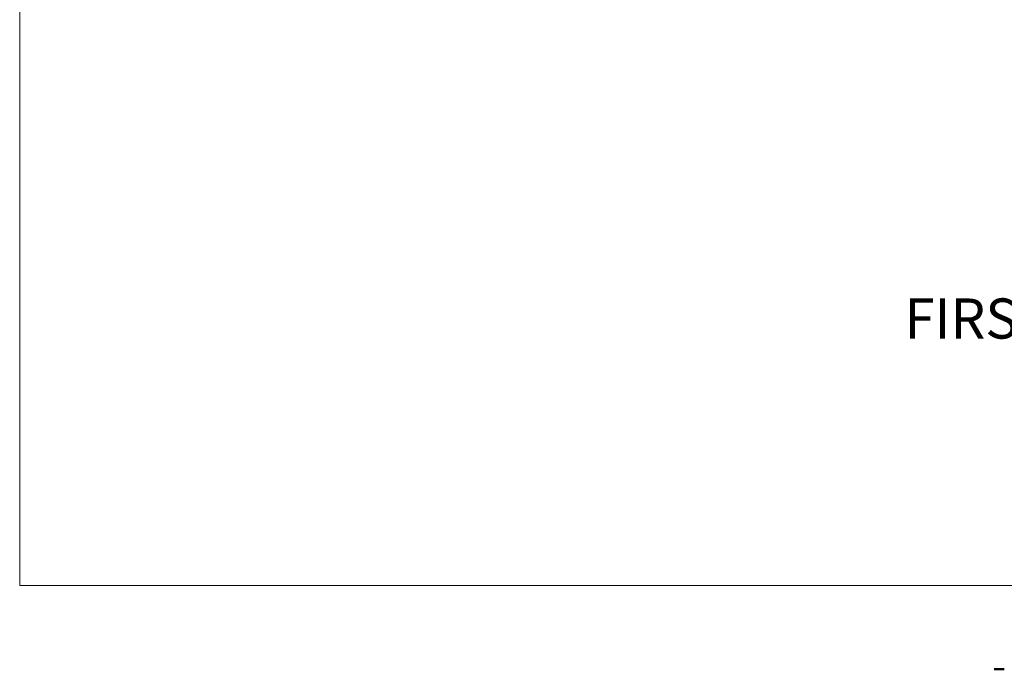
# Model space of a CAD drawing. Units: inches. Extents: x 1901 to 2863, y 888 to 2433.
# Tile 1 of 91: x 1901 to 2343, y 924 to 1216. Entities that reach past the tile are written whole.
import ezdxf

# ---------------------------------------------------------------- set-up
doc = ezdxf.new("R2010")
doc.units = ezdxf.units.IN
for name, color, linetype, lineweight in [('A-ANNO-TEXT', 7, 'Continuous', 35), ('A-FLOR-FIXT', 9, 'Continuous', 18), ('A-WALL', 7, 'Continuous', 50), ('A-WALL-PATT', 8, 'Continuous', 13)]:
    doc.layers.add(name, color=color, linetype=linetype, lineweight=lineweight)
doc.styles.get("Standard").update_dxf_attribs({"font": 'arial.ttf'})

msp = doc.modelspace()

# ---------------------------------------------------------------- hatches: boundary and pattern name
at = {"layer": 'A-WALL-PATT'}
h = msp.add_hatch(dxfattribs=at)
h.set_pattern_fill('ANSI32', color=256)
h.paths.add_polyline_path([(2192.5, 2274.13), (2141.26, 2274.13), (2141.26, 2269.63), (2192.5, 2269.63)])
h.paths.add_polyline_path([(2259.93, 2274.13), (2216.5, 2274.13), (2216.5, 2269.63), (2255.43, 2269.63), (2255.43, 2214.63), (2250.81, 2214.63), (2250.81, 2210.13), (2259.93, 2210.13), (2259.93, 2215.13), (2271.76, 2215.13), (2271.76, 2217.38), (2271.76, 2219.63), (2259.93, 2219.63)])
h.paths.add_polyline_path([(2171.43, 2269.63), (2166.93, 2269.63), (2166.93, 2219.63), (2121.24, 2219.63), (2121.24, 2215.13), (2166.93, 2215.13), (2166.93, 2083.13), (2161.81, 2083.13), (2161.81, 2078.63), (2171.43, 2078.63), (2177, 2078.63), (2177, 2080.88), (2177, 2083.13), (2171.43, 2083.13), (2171.43, 2210.13), (2230.91, 2210.13), (2230.91, 2212.38), (2230.91, 2214.63), (2171.43, 2214.63)])
h.paths.add_polyline_path([(2117.26, 2274.13), (2089.43, 2274.13), (2089.43, 2219.63), (2081.14, 2219.63), (2081.14, 2215.13), (2089.43, 2215.13), (2098, 2215.13), (2098, 2217.38), (2098, 2219.63), (2093.93, 2219.63), (2093.93, 2269.63), (2117.26, 2269.63), (2117.26, 2271.88)])
h.paths.add_polyline_path([(2343.43, 2219.63), (2329.29, 2219.63), (2329.29, 2215.13), (2338.93, 2215.13), (2338.93, 2184.74), (2343.43, 2184.74)])
h.paths.add_polyline_path([(2338.93, 2083.13), (2329.29, 2083.13), (2208.97, 2083.13), (2208.97, 2078.63), (2338.93, 2078.63)])
h.paths.add_polyline_path([(2343.43, 2136.74), (2338.93, 2136.74), (2338.93, 1872.63), (2343.43, 1872.63)])
h.paths.add_polyline_path([(2343.43, 1863.63), (2397.68, 1863.63), (2397.68, 1821.63), (2384.14, 1821.63), (2384.14, 1812.63), (2418.33, 1812.63), (2418.33, 1817.13), (2418.33, 1821.63), (2406.68, 1821.63), (2406.68, 1863.63), (2459.5, 1863.63), (2459.5, 1821.63), (2447.14, 1821.63), (2447.14, 1812.63), (2459.5, 1812.63), (2468.5, 1812.63), (2468.5, 1872.63), (2394.43, 1872.63), (2334.43, 1872.63), (2334.43, 1812.63), (2343.43, 1812.63), (2353.25, 1812.63), (2353.25, 1821.63), (2343.43, 1821.63)])
h.paths.add_polyline_path([(2510.01, 1872.63), (2468.5, 1872.63), (2468.5, 1868.13), (2510.01, 1868.13)])
h.paths.add_polyline_path([(2514.01, 1817.13), (2468.5, 1817.13), (2468.5, 1812.63), (2482.11, 1812.63), (2482.11, 1800.61), (2486.61, 1800.61), (2486.61, 1812.63), (2514.01, 1812.63)])
h.paths.add_polyline_path([(2299.25, 1814.88), (2299.25, 1817.13), (2295.93, 1817.13), (2295.93, 1854.17), (2293.68, 1854.17), (2291.43, 1854.17), (2291.43, 1817.13), (2266.11, 1817.13), (2266.11, 1812.63), (2299.25, 1812.63)])
h.paths.add_polyline_path([(2218.11, 1817.13), (2206.46, 1817.13), (2171.43, 1817.13), (2171.43, 1949.13), (2190.1, 1949.13), (2190.1, 1953.63), (2163.47, 1953.63), (2163.47, 1949.13), (2166.93, 1949.13), (2166.93, 1817.13), (2114.3, 1817.13), (2114.3, 1812.63), (2218.11, 1812.63)])
h.paths.add_polyline_path([(2029.43, 1970.92), (2024.93, 1970.92), (2024.93, 1912.72), (2029.43, 1912.72)])
h.paths.add_polyline_path([(2132.3, 1953.63), (2113.93, 1953.63), (2113.93, 1975.89), (2111.68, 1975.89), (2109.43, 1975.89), (2109.43, 1953.63), (2029.43, 1953.63), (2029.43, 1949.13), (2132.3, 1949.13)])
h.paths.add_polyline_path([(2029.43, 1853.61), (2029.31, 1853.61), (2029.31, 1853.61), (2029.43, 1853.61), (2029.43, 1864.72), (2024.93, 1864.72), (2024.93, 1812.63), (2066.3, 1812.63), (2066.3, 1814.88), (2066.3, 1817.13), (2029.43, 1817.13)])
h.paths.add_polyline_path([(2122.93, 2010.09), (2120.68, 2010.09), (2118.43, 2010.09), (2118.43, 2006.13), (2029.43, 2006.13), (2029.43, 2001.63), (2109.43, 2001.63), (2109.43, 1998.04), (2113.93, 1998.04), (2113.93, 2001.63), (2122.93, 2001.63)])
h.paths.add_polyline_path([(2029.43, 2031.38), (2024.93, 2031.38), (2024.93, 1994.92), (2027.18, 1994.92), (2029.43, 1994.92)])
h.paths.add_polyline_path([(2029.43, 2136.74), (2024.93, 2136.74), (2024.93, 2067.38), (2027.18, 2067.38), (2029.43, 2067.38)])
h.paths.add_polyline_path([(2125.62, 2083.13), (2029.43, 2083.13), (2029.43, 2078.63), (2118.43, 2078.63), (2118.43, 2030.71), (2122.93, 2030.71), (2122.93, 2078.63), (2125.62, 2078.63)])
h.paths.add_polyline_path([(2029.43, 2215.13), (2040.47, 2215.13), (2040.47, 2217.38), (2040.47, 2219.63), (2024.93, 2219.63), (2024.93, 2184.74), (2029.43, 2184.74), (2029.43, 2187.78)])
h.paths.add_polyline_path([(2686.43, 2274.13), (2659.28, 2274.13), (2659.28, 2269.63), (2681.93, 2269.63), (2681.93, 2219.63), (2676.82, 2219.63), (2676.82, 2215.13), (2681.93, 2215.13), (2697.01, 2215.13), (2697.01, 2217.38), (2697.01, 2219.63), (2686.43, 2219.63)])
h.paths.add_polyline_path([(2609.93, 2269.63), (2635.28, 2269.63), (2635.28, 2274.13), (2571.43, 2274.13), (2571.43, 2269.63), (2605.43, 2269.63), (2605.43, 2214.63), (2549.1, 2214.63), (2549.1, 2210.13), (2605.43, 2210.13), (2605.43, 2083.13), (2601.01, 2083.13), (2601.01, 2080.88), (2601.01, 2078.63), (2609.93, 2078.63), (2616.16, 2078.63), (2616.16, 2080.88), (2616.16, 2083.13), (2609.93, 2083.13), (2609.93, 2215.13), (2651.46, 2215.13), (2651.46, 2217.38), (2651.46, 2219.63), (2609.93, 2219.63)])
h.paths.add_polyline_path([(2521.43, 2269.63), (2547.43, 2269.63), (2547.43, 2271.88), (2547.43, 2274.13), (2516.93, 2274.13), (2516.93, 2219.63), (2506.41, 2219.63), (2506.41, 2215.13), (2516.93, 2215.13), (2516.93, 2210.13), (2525.4, 2210.13), (2525.4, 2212.38), (2525.4, 2214.63), (2521.43, 2214.63)])
h.paths.add_polyline_path([(2456.01, 2219.63), (2439.43, 2219.63), (2439.43, 2187.89), (2443.93, 2187.89), (2443.93, 2215.13), (2456.01, 2215.13)])
h.paths.add_polyline_path([(2752.93, 2219.63), (2739.48, 2219.63), (2739.48, 2215.13), (2748.43, 2215.13), (2748.43, 2187.89), (2752.93, 2187.89)])
h.paths.add_polyline_path([(2752.93, 2139.89), (2748.43, 2139.89), (2748.43, 2083.13), (2648.42, 2083.13), (2648.42, 2078.63), (2654.93, 2078.63), (2654.93, 2039.44), (2659.43, 2039.44), (2659.43, 2078.63), (2748.43, 2078.63), (2748.43, 2063.43), (2752.93, 2063.43)])
h.paths.add_polyline_path([(2752.93, 2010.63), (2659.43, 2010.63), (2659.43, 2015.65), (2654.93, 2015.65), (2654.93, 2010.63), (2605.43, 2010.63), (2605.43, 1920.97), (2609.93, 1920.97), (2609.93, 2006.13), (2748.43, 2006.13), (2748.43, 1982.47), (2752.93, 1982.47)])
h.paths.add_polyline_path([(2752.93, 2027.43), (2748.43, 2027.43), (2748.43, 2010.63), (2752.93, 2010.63)])
h.paths.add_polyline_path([(2748.43, 1886.13), (2609.93, 1886.13), (2609.93, 1889.72), (2605.43, 1889.72), (2605.43, 1861.26), (2609.93, 1861.26), (2609.93, 1881.63), (2748.43, 1881.63)])
h.paths.add_polyline_path([(2456.86, 2228.83), (2498.4, 2228.83), (2498.4, 2247.49), (2456.86, 2247.49)], flags=9)
h.paths.add_polyline_path([(2038.6, 2237.42), (2080.17, 2237.42), (2080.17, 2256.08), (2038.6, 2256.08)], flags=9)
h.paths.add_polyline_path([(2292.01, 1062.39), (2539.93, 1062.39), (2539.93, 1099.49), (2292.01, 1099.49)], flags=9)
h.paths.add_polyline_path([(2424.91, 1832.25), (2448.51, 1832.25), (2448.51, 1846.68), (2424.91, 1846.68)], flags=25)
h.paths.add_polyline_path([(2359.08, 1832.25), (2382.68, 1832.25), (2382.68, 1846.68), (2359.08, 1846.68)], flags=25)
h.paths.add_polyline_path([(2352.9, 1684.8), (2367.54, 1684.8), (2367.54, 1697.17), (2352.9, 1697.17)], flags=9)
h.paths.add_polyline_path([(2079.29, 1755.83), (2169.02, 1755.83), (2169.02, 1774.37), (2079.29, 1774.37)], flags=9)
h.paths.add_polyline_path([(2404.09, 1373.86), (2404.09, 1463.59), (2385.54, 1463.59), (2385.54, 1373.86)], flags=9)
h.paths.add_polyline_path([(2268.09, 2236.37), (2309.64, 2236.37), (2309.64, 2255.03), (2268.09, 2255.03)], flags=9)
h.paths.add_polyline_path([(2575.96, 1700.95), (2665.7, 1700.95), (2665.7, 1719.5), (2575.96, 1719.5)], flags=9)
h.paths.add_polyline_path([(2302.96, 1878.47), (2329.52, 1878.47), (2329.52, 1888.78), (2302.96, 1888.78)], flags=9)
h.paths.add_polyline_path([(2097.42, 2240.58), (2126.57, 2240.58), (2126.57, 2259.23), (2097.42, 2259.23)], flags=9)
h.paths.add_polyline_path([(2208.72, 2246.12), (2237.88, 2246.12), (2237.88, 2264.78), (2208.72, 2264.78)], flags=9)
h.paths.add_polyline_path([(2038.15, 1925.96), (2076.99, 1925.96), (2076.99, 1944.62), (2038.15, 1944.62)], flags=9)
h.paths.add_polyline_path([(2239.14, 1926.67), (2288.46, 1926.67), (2288.46, 1945.33), (2239.14, 1945.33)], flags=9)
h.paths.add_polyline_path([(2175.43, 2007.33), (2212.36, 2007.33), (2212.36, 2025.99), (2175.43, 2025.99)], flags=9)
h.paths.add_polyline_path([(2225.03, 2091.79), (2263.87, 2091.79), (2263.87, 2110.45), (2225.03, 2110.45)], flags=9)
h.paths.add_polyline_path([(2035.4, 2098.48), (2074.24, 2098.48), (2074.24, 2117.14), (2035.4, 2117.14)], flags=9)
h.paths.add_polyline_path([(2050.1, 2029.21), (2083.26, 2029.21), (2083.26, 2047.87), (2050.1, 2047.87)], flags=9)
h.paths.add_polyline_path([(2069.68, 1956.72), (2098.83, 1956.72), (2098.83, 1975.38), (2069.68, 1975.38)], flags=25)
h.paths.add_polyline_path([(2328.62, 1753.34), (2361.66, 1753.34), (2361.66, 1771.99), (2328.62, 1771.99)], flags=9)
h.paths.add_polyline_path([(2395.16, 2060.89), (2395.16, 2140.65), (2378.68, 2140.65), (2378.68, 2060.89)], flags=9)
h.paths.add_polyline_path([(2463.73, 2059.02), (2492.89, 2059.02), (2492.89, 2077.68), (2463.73, 2077.68)], flags=9)
h.paths.add_polyline_path([(2458.03, 2181.54), (2496.87, 2181.54), (2496.87, 2200.19), (2458.03, 2200.19)], flags=9)
h.paths.add_polyline_path([(2527.58, 2243.07), (2556.73, 2243.07), (2556.73, 2261.73), (2527.58, 2261.73)], flags=9)
h.paths.add_polyline_path([(2694.46, 2232.77), (2736.03, 2232.77), (2736.03, 2251.42), (2694.46, 2251.42)], flags=9)
h.paths.add_polyline_path([(2637.82, 2249.22), (2666.98, 2249.22), (2666.98, 2267.88), (2637.82, 2267.88)], flags=9)
h.paths.add_polyline_path([(2623.69, 2183.54), (2662.53, 2183.54), (2662.53, 2202.2), (2623.69, 2202.2)], flags=9)
h.paths.add_polyline_path([(2691.97, 2021.5), (2725.12, 2021.5), (2725.12, 2040.16), (2691.97, 2040.16)], flags=9)
h.paths.add_polyline_path([(2621.04, 1975.91), (2662.34, 1975.91), (2662.34, 1994.57), (2621.04, 1994.57)], flags=25)
h.paths.add_polyline_path([(2479.03, 1927.62), (2519.84, 1927.62), (2519.84, 1946.28), (2479.03, 1946.28)], flags=9)
h.paths.add_polyline_path([(2670.94, 1849.08), (2716.01, 1849.08), (2716.01, 1867.73), (2670.94, 1867.73)], flags=9)
h.paths.add_polyline_path([(2523.61, 1782.96), (2550.17, 1782.96), (2550.17, 1793.26), (2523.61, 1793.26)], flags=9)
h.paths.add_polyline_path([(2450.84, 1207.33), (2492.39, 1207.33), (2492.39, 1225.99), (2450.84, 1225.99)], flags=9)
h.paths.add_polyline_path([(2527.75, 1203.84), (2556.91, 1203.84), (2556.91, 1222.5), (2527.75, 1222.5)], flags=9)
h.paths.add_polyline_path([(2639.11, 1207.2), (2668.27, 1207.2), (2668.27, 1225.86), (2639.11, 1225.86)], flags=9)
h.paths.add_polyline_path([(2692.59, 1218.97), (2734.17, 1218.97), (2734.17, 1237.62), (2692.59, 1237.62)], flags=9)
h.paths.add_polyline_path([(2669.27, 1366.33), (2708.11, 1366.33), (2708.11, 1384.99), (2669.27, 1384.99)], flags=9)
h.paths.add_polyline_path([(2463.31, 1358.03), (2502.15, 1358.03), (2502.15, 1376.69), (2463.31, 1376.69)], flags=9)
h.paths.add_polyline_path([(2494.72, 1449.96), (2531.65, 1449.96), (2531.65, 1468.62), (2494.72, 1468.62)], flags=9)
h.paths.add_polyline_path([(2675.57, 1422.16), (2708.72, 1422.16), (2708.72, 1440.81), (2675.57, 1440.81)], flags=9)
h.paths.add_polyline_path([(2685.63, 1493.89), (2714.79, 1493.89), (2714.79, 1512.55), (2685.63, 1512.55)], flags=9)
h.paths.add_polyline_path([(2686.8, 1529.91), (2725.65, 1529.91), (2725.65, 1548.57), (2686.8, 1548.57)], flags=9)
h.paths.add_polyline_path([(2503.65, 1537.99), (2552.97, 1537.99), (2552.97, 1556.65), (2503.65, 1556.65)], flags=9)
h.paths.add_polyline_path([(2291.71, 1643.5), (2318.28, 1643.5), (2318.28, 1653.81), (2291.71, 1653.81)], flags=9)
h.paths.add_polyline_path([(2450.63, 1610.52), (2477.19, 1610.52), (2477.19, 1620.82), (2450.63, 1620.82)], flags=9)
h.paths.add_polyline_path([(2359.99, 1551.81), (2422.25, 1551.81), (2422.25, 1562.12), (2359.99, 1562.12)], flags=9)
h.paths.add_polyline_path([(2280.11, 1249.01), (2321.65, 1249.01), (2321.65, 1267.66), (2280.11, 1267.66)], flags=9)
h.paths.add_polyline_path([(2164.06, 1274.23), (2193.22, 1274.23), (2193.22, 1292.89), (2164.06, 1292.89)], flags=9)
h.paths.add_polyline_path([(2118.21, 1277.69), (2151.25, 1277.69), (2151.25, 1296.35), (2118.21, 1296.35)], flags=9)
h.paths.add_polyline_path([(2031.95, 1268.53), (2073.52, 1268.53), (2073.52, 1287.19), (2031.95, 1287.19)], flags=9)
h.paths.add_polyline_path([(2050.2, 1409.08), (2089.04, 1409.08), (2089.04, 1427.74), (2050.2, 1427.74)], flags=9)
h.paths.add_polyline_path([(2243.74, 1421.03), (2282.58, 1421.03), (2282.58, 1439.69), (2243.74, 1439.69)], flags=9)
h.paths.add_polyline_path([(2190.75, 1509.77), (2231.56, 1509.77), (2231.56, 1528.43), (2190.75, 1528.43)], flags=9)
h.paths.add_polyline_path([(2058.39, 1475.42), (2091.55, 1475.42), (2091.55, 1494.07), (2058.39, 1494.07)], flags=9)
h.paths.add_polyline_path([(2062.45, 1553.09), (2091.6, 1553.09), (2091.6, 1571.75), (2062.45, 1571.75)], flags=9)
h.paths.add_polyline_path([(2219.52, 1590.37), (2266.15, 1590.37), (2266.15, 1609.02), (2219.52, 1609.02)], flags=9)
h.paths.add_polyline_path([(2041.07, 1584.19), (2079.91, 1584.19), (2079.91, 1602.85), (2041.07, 1602.85)], flags=9)
h = msp.add_hatch(dxfattribs=at)
h.set_pattern_fill('ANSI32', color=256)
h.paths.add_polyline_path([(2443.93, 2139.89), (2439.43, 2139.89), (2439.43, 2069.35), (2441.68, 2069.35), (2443.93, 2069.35), (2443.93, 2078.63), (2521.93, 2078.63), (2521.93, 2075.07), (2524.18, 2075.07), (2526.43, 2075.07), (2526.43, 2078.63), (2571.75, 2078.63), (2571.75, 2080.88), (2571.75, 2083.13), (2443.93, 2083.13)])
h.paths.add_polyline_path([(2526.43, 2054.63), (2524.18, 2054.63), (2521.93, 2054.63), (2521.93, 2030.63), (2443.93, 2030.63), (2443.93, 2045.35), (2439.43, 2045.35), (2439.43, 1983.87), (2443.93, 1983.87), (2443.93, 2026.13), (2521.93, 2026.13), (2526.43, 2026.13)])
h.paths.add_polyline_path([(2443.93, 1923.87), (2439.43, 1923.87), (2439.43, 1872.63), (2443.93, 1872.63)])
h.paths.add_polyline_path([(2636.23, 1766.13), (2609.93, 1766.13), (2609.93, 1779.79), (2605.43, 1779.79), (2605.43, 1766.13), (2486.61, 1766.13), (2486.61, 1770.67), (2482.11, 1770.67), (2482.11, 1766.13), (2482.11, 1761.63), (2636.23, 1761.63), (2636.23, 1763.88)])
h.paths.add_polyline_path([(2519.54, 1663.38), (2519.54, 1665.63), (2494.93, 1665.63), (2481.83, 1665.63), (2481.83, 1663.38), (2481.83, 1661.13), (2490.43, 1661.13), (2490.43, 1640.16), (2494.93, 1640.16), (2494.93, 1661.13), (2519.54, 1661.13)])
h.paths.add_polyline_path([(2443.93, 1712.13), (2443.93, 1716.63), (2414.46, 1716.63), (2414.46, 1712.13), (2439.43, 1712.13), (2439.43, 1545.51), (2443.93, 1545.51), (2443.93, 1661.13), (2448.47, 1661.13), (2448.47, 1665.63), (2443.93, 1665.63)])
h.paths.add_polyline_path([(2343.43, 1712.13), (2365.52, 1712.13), (2365.52, 1714.38), (2365.52, 1716.63), (2333.87, 1716.63), (2333.87, 1714.38), (2333.87, 1712.13), (2338.93, 1712.13), (2338.93, 1575.63), (2338.93, 1545.51), (2343.43, 1545.51), (2343.43, 1547.51), (2343.43, 1580.13)])
h.paths.add_polyline_path([(2752.93, 1665.63), (2579.54, 1665.63), (2579.54, 1661.13), (2615.93, 1661.13), (2615.93, 1529.13), (2598.93, 1529.13), (2598.93, 1524.63), (2623.13, 1524.63), (2623.13, 1526.88), (2623.13, 1529.13), (2620.43, 1529.13), (2620.43, 1661.13), (2748.43, 1661.13), (2748.43, 1633.5), (2752.93, 1633.5)])
h.paths.add_polyline_path([(2752.93, 1419.93), (2748.43, 1419.93), (2748.43, 1400.13), (2659.43, 1400.13), (2659.43, 1444.33), (2657.18, 1444.33), (2654.93, 1444.33), (2654.93, 1400.13), (2643.65, 1400.13), (2643.65, 1395.63), (2748.43, 1395.63), (2748.43, 1364.04), (2752.93, 1364.04)])
h.paths.add_polyline_path([(2752.93, 1492.88), (2748.43, 1492.88), (2748.43, 1476.63), (2667.43, 1476.63), (2667.43, 1479.71), (2665.18, 1479.71), (2662.93, 1479.71), (2662.93, 1476.63), (2654.93, 1476.63), (2654.93, 1469.54), (2659.43, 1469.54), (2659.43, 1472.13), (2748.43, 1472.13), (2748.43, 1455.93), (2752.93, 1455.93)])
h.paths.add_polyline_path([(2752.93, 1304.04), (2748.43, 1304.04), (2748.43, 1263.63), (2738.66, 1263.63), (2738.66, 1259.13), (2752.93, 1259.13)])
h.paths.add_polyline_path([(2685.93, 1259.13), (2695.49, 1259.13), (2695.49, 1261.38), (2695.49, 1263.63), (2677.84, 1263.63), (2677.84, 1261.38), (2677.84, 1259.13), (2681.43, 1259.13), (2681.43, 1203.63), (2653.28, 1203.63), (2653.28, 1199.13), (2685.93, 1199.13), (2685.93, 1203.63)])
h.paths.add_polyline_path([(2609.43, 1395.63), (2611.85, 1395.63), (2611.85, 1400.13), (2598.89, 1400.13), (2598.89, 1397.88), (2598.89, 1395.63), (2604.93, 1395.63), (2604.93, 1268.13), (2554.73, 1268.13), (2554.73, 1265.88), (2554.73, 1263.63), (2604.93, 1263.63), (2604.93, 1203.63), (2571.31, 1203.63), (2571.31, 1199.13), (2604.93, 1199.13), (2629.28, 1199.13), (2629.28, 1201.38), (2629.28, 1203.63), (2609.43, 1203.63), (2609.43, 1258.63), (2609.43, 1259.13), (2654.8, 1259.13), (2654.8, 1263.63), (2609.43, 1263.63)])
h.paths.add_polyline_path([(2443.93, 1304.04), (2439.43, 1304.04), (2439.43, 1259.13), (2443.93, 1259.13), (2456.16, 1259.13), (2456.16, 1261.38), (2456.16, 1263.63), (2443.93, 1263.63)])
h.paths.add_polyline_path([(2525.43, 1263.63), (2531.78, 1263.63), (2531.78, 1268.13), (2520.93, 1268.13), (2520.93, 1263.63), (2511.41, 1263.63), (2511.41, 1259.13), (2520.93, 1259.13), (2520.93, 1199.13), (2547.31, 1199.13), (2547.31, 1201.38), (2547.31, 1203.63), (2525.43, 1203.63)])
h.paths.add_polyline_path([(2443.93, 1434.84), (2439.43, 1434.84), (2439.43, 1364.04), (2441.68, 1364.04), (2443.93, 1364.04)])
h.paths.add_polyline_path([(2567.13, 1400.13), (2443.93, 1400.13), (2443.93, 1395.63), (2567.13, 1395.63)])
h.paths.add_polyline_path([(2443.93, 1545.51), (2439.43, 1545.51), (2439.43, 1494.84), (2443.93, 1494.84)])
h.paths.add_polyline_path([(2494.93, 1553.35), (2492.68, 1553.35), (2490.43, 1553.35), (2490.43, 1524.63), (2494.93, 1524.63), (2525.94, 1524.63), (2525.94, 1526.88), (2525.94, 1529.13), (2494.93, 1529.13)])
h.paths.add_polyline_path([(2752.93, 1573.5), (2748.43, 1573.5), (2748.43, 1529.13), (2657.76, 1529.13), (2657.76, 1524.63), (2662.93, 1524.63), (2662.93, 1498.63), (2667.43, 1498.63), (2667.43, 1524.63), (2748.43, 1524.63), (2748.43, 1516.88), (2752.93, 1516.88)])
h.paths.add_polyline_path([(2038.6, 2237.42), (2080.17, 2237.42), (2080.17, 2256.08), (2038.6, 2256.08)], flags=9)
h.paths.add_polyline_path([(2292.01, 1062.39), (2539.93, 1062.39), (2539.93, 1099.49), (2292.01, 1099.49)], flags=9)
h.paths.add_polyline_path([(2424.91, 1832.25), (2448.51, 1832.25), (2448.51, 1846.68), (2424.91, 1846.68)], flags=9)
h.paths.add_polyline_path([(2359.08, 1832.25), (2382.68, 1832.25), (2382.68, 1846.68), (2359.08, 1846.68)], flags=9)
h.paths.add_polyline_path([(2352.9, 1684.8), (2367.54, 1684.8), (2367.54, 1697.17), (2352.9, 1697.17)], flags=9)
h.paths.add_polyline_path([(2079.29, 1755.83), (2169.02, 1755.83), (2169.02, 1774.37), (2079.29, 1774.37)], flags=9)
h.paths.add_polyline_path([(2404.09, 1373.86), (2404.09, 1463.59), (2385.54, 1463.59), (2385.54, 1373.86)], flags=9)
h.paths.add_polyline_path([(2268.09, 2236.37), (2309.64, 2236.37), (2309.64, 2255.03), (2268.09, 2255.03)], flags=9)
h.paths.add_polyline_path([(2575.96, 1700.95), (2665.7, 1700.95), (2665.7, 1719.5), (2575.96, 1719.5)], flags=9)
h.paths.add_polyline_path([(2302.96, 1878.47), (2329.52, 1878.47), (2329.52, 1888.78), (2302.96, 1888.78)], flags=9)
h.paths.add_polyline_path([(2097.42, 2240.58), (2126.57, 2240.58), (2126.57, 2259.23), (2097.42, 2259.23)], flags=9)
h.paths.add_polyline_path([(2208.72, 2246.12), (2237.88, 2246.12), (2237.88, 2264.78), (2208.72, 2264.78)], flags=9)
h.paths.add_polyline_path([(2038.15, 1925.96), (2076.99, 1925.96), (2076.99, 1944.62), (2038.15, 1944.62)], flags=9)
h.paths.add_polyline_path([(2239.14, 1926.67), (2288.46, 1926.67), (2288.46, 1945.33), (2239.14, 1945.33)], flags=9)
h.paths.add_polyline_path([(2175.43, 2007.33), (2212.36, 2007.33), (2212.36, 2025.99), (2175.43, 2025.99)], flags=9)
h.paths.add_polyline_path([(2225.03, 2091.79), (2263.87, 2091.79), (2263.87, 2110.45), (2225.03, 2110.45)], flags=9)
h.paths.add_polyline_path([(2035.4, 2098.48), (2074.24, 2098.48), (2074.24, 2117.14), (2035.4, 2117.14)], flags=9)
h.paths.add_polyline_path([(2050.1, 2029.21), (2083.26, 2029.21), (2083.26, 2047.87), (2050.1, 2047.87)], flags=9)
h.paths.add_polyline_path([(2069.68, 1956.72), (2098.83, 1956.72), (2098.83, 1975.38), (2069.68, 1975.38)], flags=9)
h.paths.add_polyline_path([(2328.62, 1753.34), (2361.66, 1753.34), (2361.66, 1771.99), (2328.62, 1771.99)], flags=9)
h.paths.add_polyline_path([(2395.16, 2060.89), (2395.16, 2140.65), (2378.68, 2140.65), (2378.68, 2060.89)], flags=9)
h.paths.add_polyline_path([(2463.73, 2059.02), (2492.89, 2059.02), (2492.89, 2077.68), (2463.73, 2077.68)], flags=9)
h.paths.add_polyline_path([(2458.03, 2181.54), (2496.87, 2181.54), (2496.87, 2200.19), (2458.03, 2200.19)], flags=9)
h.paths.add_polyline_path([(2456.86, 2228.83), (2498.4, 2228.83), (2498.4, 2247.49), (2456.86, 2247.49)], flags=9)
h.paths.add_polyline_path([(2527.58, 2243.07), (2556.73, 2243.07), (2556.73, 2261.73), (2527.58, 2261.73)], flags=9)
h.paths.add_polyline_path([(2694.46, 2232.77), (2736.03, 2232.77), (2736.03, 2251.42), (2694.46, 2251.42)], flags=9)
h.paths.add_polyline_path([(2637.82, 2249.22), (2666.98, 2249.22), (2666.98, 2267.88), (2637.82, 2267.88)], flags=9)
h.paths.add_polyline_path([(2623.69, 2183.54), (2662.53, 2183.54), (2662.53, 2202.2), (2623.69, 2202.2)], flags=9)
h.paths.add_polyline_path([(2691.97, 2021.5), (2725.12, 2021.5), (2725.12, 2040.16), (2691.97, 2040.16)], flags=9)
h.paths.add_polyline_path([(2621.04, 1975.91), (2662.34, 1975.91), (2662.34, 1994.57), (2621.04, 1994.57)], flags=9)
h.paths.add_polyline_path([(2479.03, 1927.62), (2519.84, 1927.62), (2519.84, 1946.28), (2479.03, 1946.28)], flags=9)
h.paths.add_polyline_path([(2670.94, 1849.08), (2716.01, 1849.08), (2716.01, 1867.73), (2670.94, 1867.73)], flags=9)
h.paths.add_polyline_path([(2523.61, 1782.96), (2550.17, 1782.96), (2550.17, 1793.26), (2523.61, 1793.26)], flags=9)
h.paths.add_polyline_path([(2450.84, 1207.33), (2492.39, 1207.33), (2492.39, 1225.99), (2450.84, 1225.99)], flags=9)
h.paths.add_polyline_path([(2527.75, 1203.84), (2556.91, 1203.84), (2556.91, 1222.5), (2527.75, 1222.5)], flags=9)
h.paths.add_polyline_path([(2639.11, 1207.2), (2668.27, 1207.2), (2668.27, 1225.86), (2639.11, 1225.86)], flags=9)
h.paths.add_polyline_path([(2692.59, 1218.97), (2734.17, 1218.97), (2734.17, 1237.62), (2692.59, 1237.62)], flags=9)
h.paths.add_polyline_path([(2669.27, 1366.33), (2708.11, 1366.33), (2708.11, 1384.99), (2669.27, 1384.99)], flags=25)
h.paths.add_polyline_path([(2463.31, 1358.03), (2502.15, 1358.03), (2502.15, 1376.69), (2463.31, 1376.69)], flags=9)
h.paths.add_polyline_path([(2494.72, 1449.96), (2531.65, 1449.96), (2531.65, 1468.62), (2494.72, 1468.62)], flags=9)
h.paths.add_polyline_path([(2675.57, 1422.16), (2708.72, 1422.16), (2708.72, 1440.81), (2675.57, 1440.81)], flags=25)
h.paths.add_polyline_path([(2685.63, 1493.89), (2714.79, 1493.89), (2714.79, 1512.55), (2685.63, 1512.55)], flags=9)
h.paths.add_polyline_path([(2686.8, 1529.91), (2725.65, 1529.91), (2725.65, 1548.57), (2686.8, 1548.57)], flags=25)
h.paths.add_polyline_path([(2503.65, 1537.99), (2552.97, 1537.99), (2552.97, 1556.65), (2503.65, 1556.65)], flags=9)
h.paths.add_polyline_path([(2291.71, 1643.5), (2318.28, 1643.5), (2318.28, 1653.81), (2291.71, 1653.81)], flags=9)
h.paths.add_polyline_path([(2450.63, 1610.52), (2477.19, 1610.52), (2477.19, 1620.82), (2450.63, 1620.82)], flags=9)
h.paths.add_polyline_path([(2359.99, 1551.81), (2422.25, 1551.81), (2422.25, 1562.12), (2359.99, 1562.12)], flags=9)
h.paths.add_polyline_path([(2280.11, 1249.01), (2321.65, 1249.01), (2321.65, 1267.66), (2280.11, 1267.66)], flags=9)
h.paths.add_polyline_path([(2164.06, 1274.23), (2193.22, 1274.23), (2193.22, 1292.89), (2164.06, 1292.89)], flags=9)
h.paths.add_polyline_path([(2118.21, 1277.69), (2151.25, 1277.69), (2151.25, 1296.35), (2118.21, 1296.35)], flags=9)
h.paths.add_polyline_path([(2031.95, 1268.53), (2073.52, 1268.53), (2073.52, 1287.19), (2031.95, 1287.19)], flags=9)
h.paths.add_polyline_path([(2050.2, 1409.08), (2089.04, 1409.08), (2089.04, 1427.74), (2050.2, 1427.74)], flags=9)
h.paths.add_polyline_path([(2243.74, 1421.03), (2282.58, 1421.03), (2282.58, 1439.69), (2243.74, 1439.69)], flags=9)
h.paths.add_polyline_path([(2190.75, 1509.77), (2231.56, 1509.77), (2231.56, 1528.43), (2190.75, 1528.43)], flags=9)
h.paths.add_polyline_path([(2058.39, 1475.42), (2091.55, 1475.42), (2091.55, 1494.07), (2058.39, 1494.07)], flags=9)
h.paths.add_polyline_path([(2062.45, 1553.09), (2091.6, 1553.09), (2091.6, 1571.75), (2062.45, 1571.75)], flags=9)
h.paths.add_polyline_path([(2219.52, 1590.37), (2266.15, 1590.37), (2266.15, 1609.02), (2219.52, 1609.02)], flags=9)
h.paths.add_polyline_path([(2041.07, 1584.19), (2079.91, 1584.19), (2079.91, 1602.85), (2041.07, 1602.85)], flags=9)

# ---------------------------------------------------------------- linework, layer by layer
at = {"layer": 'A-FLOR-FIXT'}
msp.add_lwpolyline([(1901.45, 2433.12), (2863.43, 2433.12), (2863.43, 961.82), (1901.45, 961.82)], close=True, dxfattribs=at)
at = {"layer": 'A-WALL'}
msp.add_line((2338.93, 924.21), (2343.43, 924.21), dxfattribs=at)

# ---------------------------------------------------------------- texts
at = {"layer": 'A-ANNO-TEXT', "insert": (2298.57, 1090.54), "char_height": 18, "attachment_point": 1}
msp.add_mtext_dynamic_manual_height_columns('FIRST FLOOR PLAN', width=549.622, gutter_width=12.5, heights=[0], dxfattribs=at)

doc.saveas('drawing.dxf')
